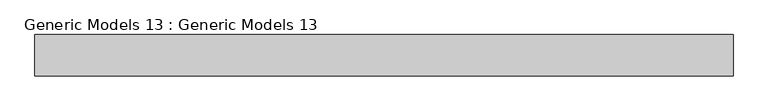
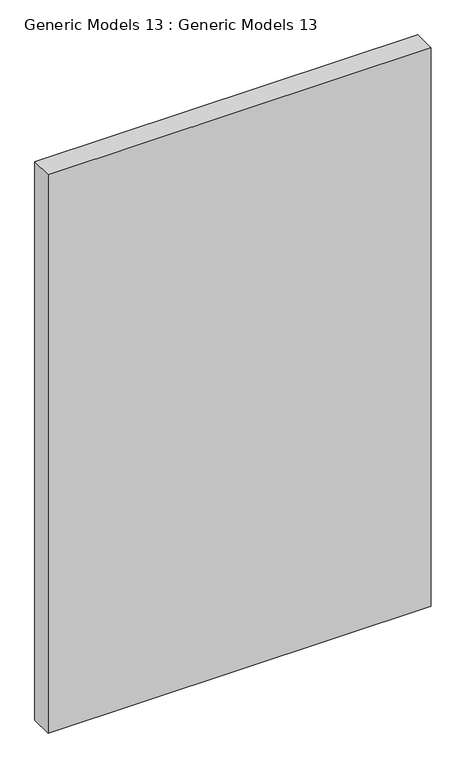
"""IFC4 building model written with IfcOpenShell, lengths in millimetres: proxy geometry, Generic Models 13 : Generic Models 13."""

from ifc_helpers import new_model, si_unit, origin, origin_with_axes, place, context, project, spatial, polyline, outline, extrude, source, transform, mapped, element, save


def generic_models_13_generic_models_13_60817c59(model_context):
    return source(origin(), model_context, "Body", "SweptSolid", [
        extrude(outline(polyline([(-26243.0645004, 6176.3256148), (-28814.8145004, 6176.3256148), (-28814.8145004, 6328.7256148), (-26243.0645004, 6328.7256148), (-26243.0645004, 6176.3256148)])), origin_with_axes(), (0.0, 0.0, 1.0), 3962.4),
    ])


if __name__ == "__main__":
    model = new_model("IFC4")
    model_context = context("Model", 3, world=origin())
    ifc_project = project(units=[si_unit("LENGTHUNIT", "METRE", prefix="MILLI")], contexts=[model_context])
    site = spatial("IfcSite", under=ifc_project)
    building = spatial("IfcBuilding", under=site)
    placement = place(None, origin())
    generic_models_13_generic_models_13_shape = generic_models_13_generic_models_13_60817c59(model_context)
    element("IfcBuildingElementProxy", 1, Name="Generic Models 13 : Generic Models 13", ObjectType="Generic Models 13 : Generic Models 13", at=placement, inside=building, context=model_context, shape_type="MappedRepresentation", body=[
        mapped(generic_models_13_generic_models_13_shape, transform((0.0, 0.0, 0.0), x_axis=(1.0, 0.0, 0.0), y_axis=(0.0, 1.0, 0.0), z_axis=(0.0, 0.0, 1.0))),
    ])
    save(model, "model.ifc")
